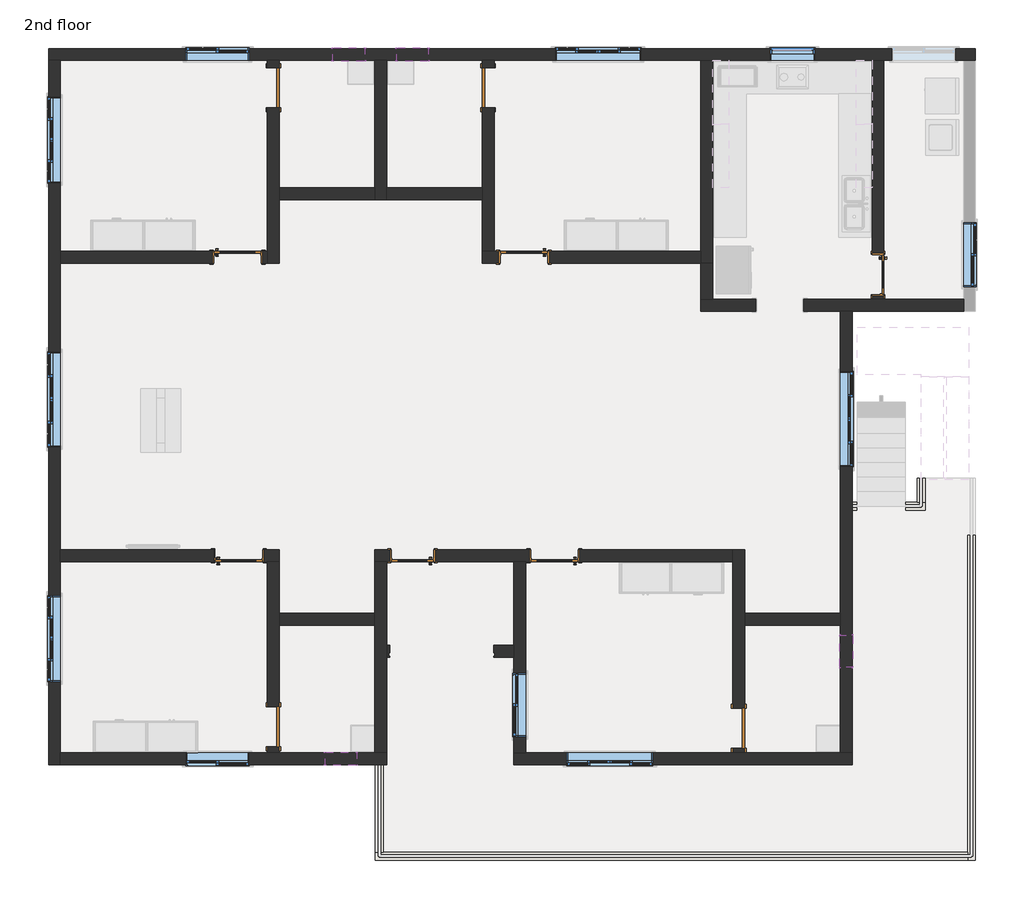
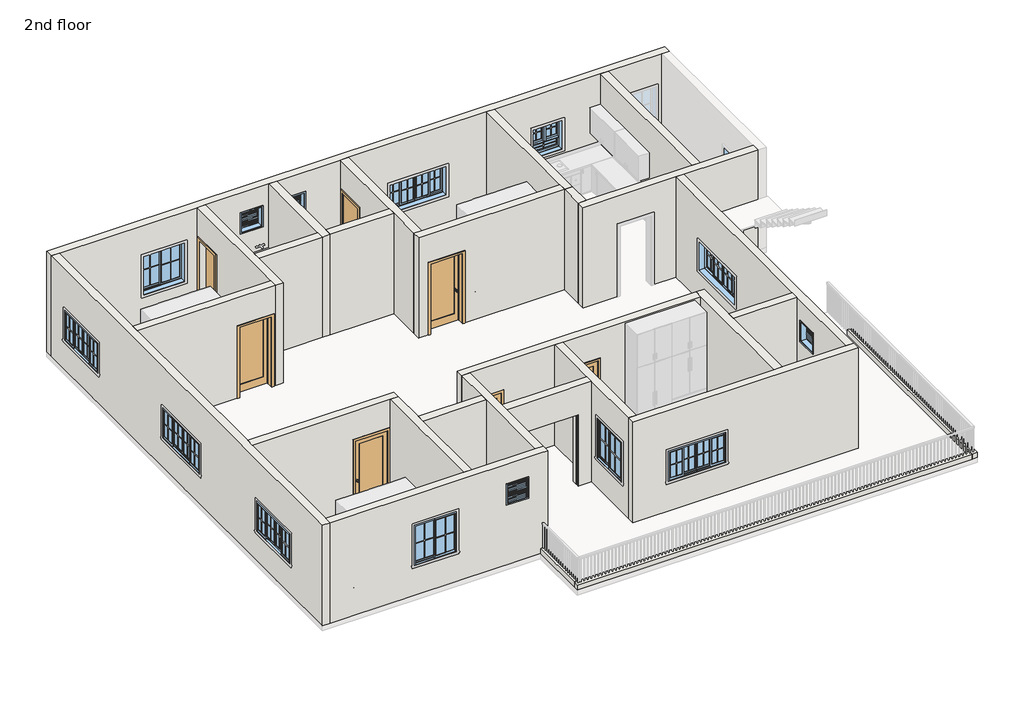
# One storey, part 1 of 4: 31 walls, 15 windows, 10 doors.
# Revit data of these elements (continued)
# Type "Window-Sliding-Four : 65\" x 36\"" (continued)
#   Interior Trim = Trim-Window-Interior-Flat : Picture Frame
#   Interior Frame Material = Wood - Stained
#   Glass Panel Material = Glass
#   Exterior Trim Material = Clad - White
#   Exterior Trim = Trim-Window-Exterior-Flat : with Sill
#   Exterior Frame Material = Clad - White
#   Wall Closure = (empty or 0)
# Type "Window-Sliding-Four : 72\" x 36\""
#   Type Mark = "20"
#   Fire Rating = "0.5h"
#   Assembly Code = "B2020100"
#   Analytic Construction = "Double glazing - domestic"
#   Window Inset [instance default] = 0' - 0"
#   Wall Thickness [instance default] = 0' - 6"
#   Visual Light Transmittance = 0.81
#   Thermal Resistance (R) = 1.8146 (h·ft²·°F)/BTU
#   Solar Heat Gain Coefficient = 0.76
#   Interior Wall Closure [instance default] = 0' - 2 19/32"
#   Heat Transfer Coefficient (U) = 0.5511 BTU/(h·ft²·°F)
#   Frame Extension [instance default] = 0' - 0 1/4"
#   Exterior Wall Closure [instance default] = 0' - 1 1/4"
#   Rough Width = 6' - 0 1/2"
#   Rough Height = 3' - 0 1/2"
#   Height = 3' - 0"
#   Extension Jamb [instance default] = 0' - 2 3/4"
#   Default Sill Height = 3' - 0"
#   Width = 6' - 0"
#   Middle Muntin Visibility = yes
#   Interior Trim Visibility [instance default] = yes
#   Indicator Visibility [instance default] = yes
#   Exterior Trim Visibility [instance default] = yes
#   Side Muntin Visibility = yes
#   Extension Jamb Visibility [instance default] = yes
#   Interior Trim Material = Wood - Stained
#   Muntin Pattern = Muntin Pattern_2x2 : Muntin Pattern_2x2
#   Interior Trim = Trim-Window-Interior-Flat : Picture Frame
#   Interior Frame Material = Wood - Stained
#   Glass Panel Material = Glass
#   Exterior Trim Material = Clad - White
#   Exterior Trim = Trim-Window-Exterior-Flat : with Sill
#   Exterior Frame Material = Clad - White
#   Wall Closure = (empty or 0)
# Element 1 (IfcDoor, "Door-Interior-Single-1_Panel-Wood : 30\" x 84\"")
#   Swing Angle = 90.00°
#   Phase Created = New Construction
#   Materials on its faces: "Cherry", "Aluminum"
# Elements 2, 3, 4, 5 (IfcDoor, "Door-Interior-Single-1_Panel-Wood : 36\" x 84\"")
#   Swing Angle = 90.00°
#   Phase Created = New Construction
#   Materials on its faces: "Cherry", "Aluminum"
# Element 6 (IfcDoor, "Door-Interior-Single-Full Glass-Wood : 32\" x 84\"")
#   Swing Angle = 90.00°
#   Show Grill = yes
#   Phase Created = New Construction
#   Materials on its faces: "Cherry", "Aluminum", "Glass"
# Elements 7, 8, 9, 10 (IfcDoor, "Single-Flush : 30\" x 84\"")
#   Phase Created = New Construction
#   Materials on its faces: "Door - Frame", "Door - Panel"
# Elements 11, 12, 13, 14, 15, 16 (IfcWall, "Generic - 6\"")
#   Top Offset = 0' - 0"
#   Base Offset = 0' - 0"
#   Unconnected Height = 0' - 6"
#   wall height = 0' - 6"
#   Phase Created = New Construction
#   Base Constraint = 2nd floor
#   Materials on its faces: "Default Wall"
# Elements 17, 18, 19, 20, 21, 22, 23, 24, 25, 26, 27, 28, 29, 30, 31, 32, 33, 34, 35, 36, 37, 38, 39, 40, 41 (IfcWall, "Generic - 9\"")
#   Top Offset = 0' - 0"
#   Base Offset = 0' - 0"
#   wall height = 10' - 0"
#   Phase Created = New Construction
#   Base Constraint = 2nd floor
#   Top Constraint = terrace
#   Materials on its faces: "Default Wall"
# Element 42 (IfcWindow, "Window-Casement-Double-Awning : 34\" x 36\"")
#   Mark = "54"
#   Window Inset = 0' - 0"
#   Interior Wall Closure = 0' - 2 1/4"
#   Frame Extension = 0' - 0 1/4"
#   Exterior Wall Closure = 0' - 1 1/4"
#   Interior Trim Visibility = yes
#   Exterior Trim Visibility = yes
#   Phase Created = New Construction
#   Materials on its faces: "Wood - Stained", "Glass", "Clad - White"
# Element 43 (IfcWindow, "Window-Louvers : 24\" x 24\"")
#   Mark = "48"
#   Blade Width = 1' - 10 1/2"
#   Phase Created = New Construction
#   Materials on its faces: "Birch"
# Element 44 (IfcWindow, "Window-Louvers : 24\" x 24\"")
#   Mark = "49"
#   Blade Width = 1' - 10 1/2"
#   Phase Created = New Construction
#   Materials on its faces: "Birch"
# Element 45 (IfcWindow, "Window-Louvers : 24\" x 24\"")
#   Mark = "55"
#   Blade Width = 1' - 10 1/2"
#   Phase Created = New Construction
#   Materials on its faces: "Birch"
# Element 46 (IfcWindow, "Window-Louvers : 24\" x 24\"")
#   Mark = "56"
#   Blade Width = 1' - 10 1/2"
#   Phase Created = New Construction
#   Materials on its faces: "Birch"
# Element 47 (IfcWindow, "Window-Sliding-Double : 48\" x 48\"")
#   Mark = "45"
#   Window Inset = 0' - 0"
#   Interior Wall Closure = 0' - 2 3/4"
#   Frame Extension = 0' - 0 1/4"
#   Exterior Wall Closure = 0' - 1 1/4"
#   Interior Trim Visibility = yes
#   Indicator Visibility = yes
#   Exterior Trim Visibility = yes
#   Phase Created = New Construction
#   Materials on its faces: "Wood - Stained", "Glass", "Clad - White"
# Element 48 (IfcWindow, "Window-Sliding-Double : 48\" x 48\"")
#   Mark = "47"
#   Window Inset = 0' - 0"
#   Interior Wall Closure = 0' - 2 3/4"
#   Frame Extension = 0' - 0 1/4"
#   Exterior Wall Closure = 0' - 1 1/4"
#   Interior Trim Visibility = yes
#   Indicator Visibility = yes
#   Exterior Trim Visibility = yes
#   Phase Created = New Construction
#   Materials on its faces: "Wood - Stained", "Glass", "Clad - White"
# Element 49 (IfcWindow, "Window-Sliding-Double : 48\" x 48\"")
#   Mark = "52"
#   Window Inset = 0' - 0"
#   Interior Wall Closure = 0' - 2 3/4"
#   Frame Extension = 0' - 0 1/4"
#   Exterior Wall Closure = 0' - 1 1/4"
#   Interior Trim Visibility = yes
#   Indicator Visibility = yes
#   Exterior Trim Visibility = yes
#   Phase Created = New Construction
#   Materials on its faces: "Wood - Stained", "Glass", "Clad - White"
# Element 50 (IfcWindow, "Window-Sliding-Double : 48\" x 48\"")
#   Mark = "53"
#   Window Inset = 0' - 0"
#   Interior Wall Closure = 0' - 2 3/4"
#   Frame Extension = 0' - 0 1/4"
#   Exterior Wall Closure = 0' - 1 1/4"
#   Interior Trim Visibility = yes
#   Indicator Visibility = yes
#   Exterior Trim Visibility = yes
#   Phase Created = New Construction
#   Materials on its faces: "Wood - Stained", "Glass", "Clad - White"
# Element 51 (IfcWindow, "Window-Sliding-Four : 65\" x 36\"")
#   Mark = "41"
#   Window Inset = 0' - 0"
#   Interior Wall Closure = 0' - 2 3/4"
#   Frame Extension = 0' - 0 1/4"
#   Exterior Wall Closure = 0' - 1 1/4"
#   Interior Trim Visibility = yes
#   Indicator Visibility = yes
#   Exterior Trim Visibility = yes
#   Phase Created = New Construction
#   Materials on its faces: "Wood - Stained", "Glass", "Clad - White"
# Element 52 (IfcWindow, "Window-Sliding-Four : 65\" x 36\"")
#   Mark = "42"
#   Window Inset = 0' - 0"
#   Interior Wall Closure = 0' - 2 3/4"
#   Frame Extension = 0' - 0 1/4"
#   Exterior Wall Closure = 0' - 1 1/4"
#   Interior Trim Visibility = yes
#   Indicator Visibility = yes
#   Exterior Trim Visibility = yes
#   Phase Created = New Construction
#   Materials on its faces: "Wood - Stained", "Glass", "Clad - White"
# Element 53 (IfcWindow, "Window-Sliding-Four : 65\" x 36\"")
#   Mark = "50"
#   Window Inset = 0' - 0"
#   Interior Wall Closure = 0' - 2 3/4"
#   Frame Extension = 0' - 0 1/4"
#   Exterior Wall Closure = 0' - 1 1/4"
#   Interior Trim Visibility = yes
#   Indicator Visibility = yes
#   Exterior Trim Visibility = yes
#   Phase Created = New Construction
#   Materials on its faces: "Wood - Stained", "Glass", "Clad - White"
# Element 54 (IfcWindow, "Window-Sliding-Four : 65\" x 36\"")
#   Mark = "51"
#   Window Inset = 0' - 0"
#   Interior Wall Closure = 0' - 2 3/4"
#   Frame Extension = 0' - 0 1/4"
#   Exterior Wall Closure = 0' - 1 1/4"
#   Interior Trim Visibility = yes
#   Indicator Visibility = yes
#   Exterior Trim Visibility = yes
#   Phase Created = New Construction
#   Materials on its faces: "Wood - Stained", "Glass", "Clad - White"
# Element 55 (IfcWindow, "Window-Sliding-Four : 72\" x 36\"")
#   Mark = "43"
#   Window Inset = 0' - 0"
#   Interior Wall Closure = 0' - 2 19/32"
#   Frame Extension = 0' - 0 1/4"
#   Exterior Wall Closure = 0' - 1 1/4"
#   Interior Trim Visibility = yes
#   Indicator Visibility = yes
#   Exterior Trim Visibility = yes
#   Phase Created = New Construction
#   Materials on its faces: "Wood - Stained", "Glass", "Clad - White"
# Element 56 (IfcWindow, "Window-Sliding-Four : 72\" x 36\"")
#   Mark = "44"
#   Window Inset = 0' - 0"
#   Interior Wall Closure = 0' - 2 19/32"
#   Frame Extension = 0' - 0 1/4"
#   Exterior Wall Closure = 0' - 1 1/4"
#   Interior Trim Visibility = yes
#   Indicator Visibility = yes
#   Exterior Trim Visibility = yes
#   Phase Created = New Construction
#   Materials on its faces: "Wood - Stained", "Glass", "Clad - White"
# Materials
#   "Cherry": class "Wood", colour RGB 226 177 128, transparency 0, Description = "Prunus Serotina", Cost = 0
#   "Aluminum": class "Metal", colour RGB 247 247 247, transparency 0, Description = "Aluminum 6061", Cost = 0
#   "Door - Panel": class "Wood", colour RGB 210 159 95, transparency 0, Cost = 0
#   "Door - Frame": colour RGB 118 70 51, transparency 0, Cost = 0
#   "Wood - Stained": class "Wood", colour RGB 224 178 126, transparency 0, Cost = 0
#   "Clad - White": class "Wood", colour RGB 242 242 238, transparency 0, Cost = 0
#   "Glass": class "Glass", colour RGB 0 128 192, transparency 0.75, Description = "Soda Lime Glass", Cost = 0
#   "Birch": class "Wood", colour RGB 224 178 126, transparency 0, Description = "Betula Alleghaniensis", Cost = 0
#   "Default Wall": colour RGB 128 128 128, transparency 0, Cost = 0
